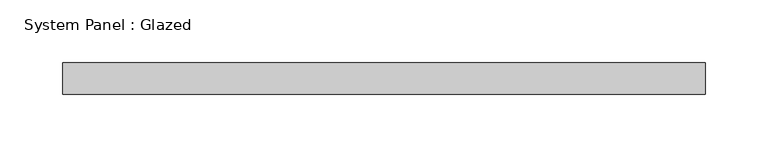
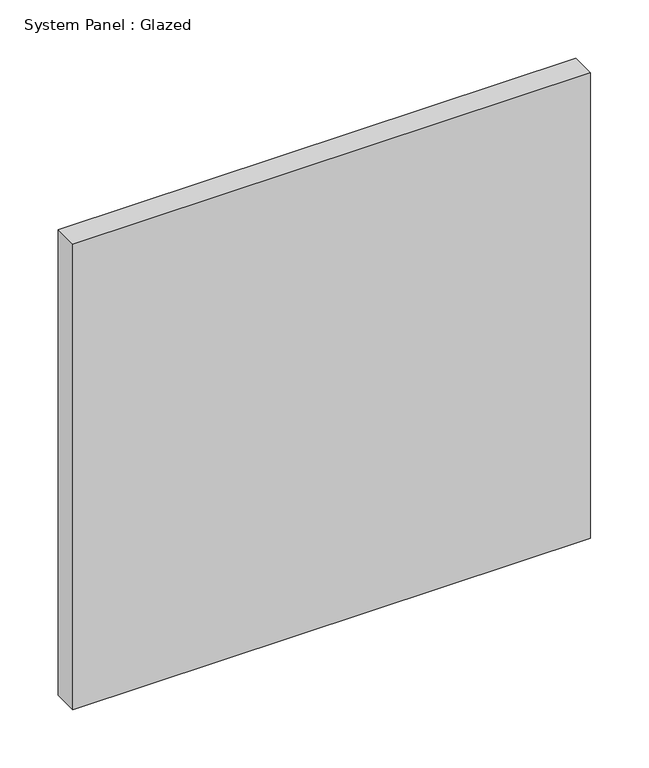
"""IFC4 building model written with IfcOpenShell, lengths in millimetres: plate geometry, System Panel : Glazed."""

from ifc_helpers import new_model, si_unit, origin, origin_with_axes, place, context, project, spatial, polyline, outline, extrude, source, transform, mapped, element, save


def system_panel_glazed_c28d2e47(model_context):
    return source(origin(), model_context, "Body", "SweptSolid", [
        extrude(outline(polyline([(257.175, 19.05), (-257.175, 19.05), (-257.175, 44.45), (257.175, 44.45), (257.175, 19.05)])), origin_with_axes(), (0.0, 0.0, 1.0), 488.6467564),
    ])


if __name__ == "__main__":
    model = new_model("IFC4")
    model_context = context("Model", 3, world=origin())
    ifc_project = project(units=[si_unit("LENGTHUNIT", "METRE", prefix="MILLI")], contexts=[model_context])
    site = spatial("IfcSite", under=ifc_project)
    building = spatial("IfcBuilding", under=site)
    placement = place(None, origin())
    system_panel_glazed_shape = system_panel_glazed_c28d2e47(model_context)
    element("IfcPlate", 1, ObjectType="System Panel : Glazed", at=placement, inside=building, context=model_context, shape_type="MappedRepresentation", body=[
        mapped(system_panel_glazed_shape, transform((0.0, 0.0, 0.0), x_axis=(1.0, 0.0, 0.0), y_axis=(0.0, 1.0, 0.0), z_axis=(0.0, 0.0, 1.0))),
    ])
    save(model, "model.ifc")

# Revit data of these elements
# Type "System Panel : Glazed"
#   Construction Type Id = "GSP4R"
#   Analytic Construction = "1/8 in Pilkington single glazing"
#   Visual Light Transmittance = 0.9
#   Solar Heat Gain Coefficient = 0.86
#   Heat Transfer Coefficient (U) = 1.18115 BTU/(h·ft²·°F)
#   Define Thermal Properties by = 1
# Element 1 (IfcPlate, "System Panel : Glazed")
#   Materials on its faces: "Glass"
# Materials
#   "Glass": class "Glass", colour RGB 0 128 192, transparency 0.75, Description = "Soda Lime Glass", Cost = 0
